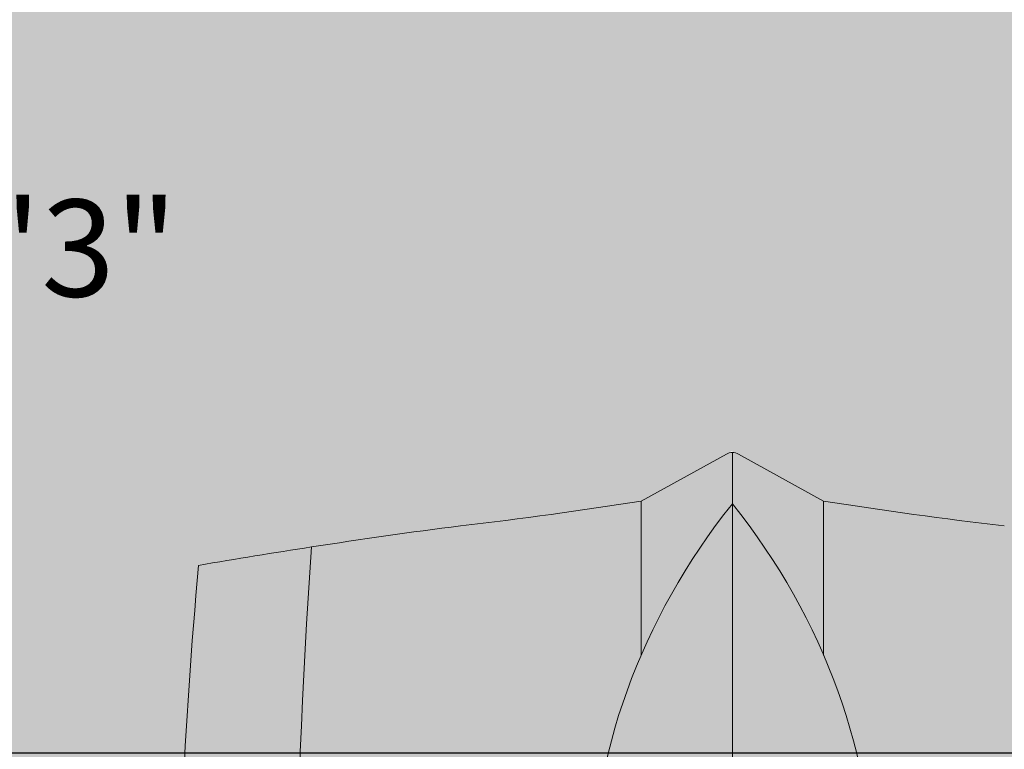
# Model space of a CAD drawing. Units: inches. Extents: x 389 to 971, y 148 to 870.
# Tile 2 of 14: x 477 to 529, y 389 to 428. Entities that reach past the tile are written whole.
import ezdxf

# ---------------------------------------------------------------- set-up
doc = ezdxf.new("R2010")
doc.units = ezdxf.units.IN
doc.header["$MEASUREMENT"] = 0
for name, color, linetype, lineweight in [('A-ANNO-DIMS', 2, 'Continuous', 18), ('A-AREA-IDEN', 7, 'Continuous', 18), ('C-VEHI', 8, 'Continuous', 13), ('L-GRND-BASE-PATT', 8, 'Continuous', 13)]:
    doc.layers.add(name, color=color, linetype=linetype, lineweight=lineweight)
doc.layers.add('C-VEHI-PATT', color=18, linetype='Continuous', lineweight=13, true_color=0x000000)
doc.layers.add('L-GRND-PATT', color=39, linetype='Continuous', lineweight=13, true_color=0x603913)
doc.styles.get("Standard").update_dxf_attribs({"font": 'arial.ttf'})
doc.dimstyles.get("Standard").update_dxf_attribs({"dimtxt": 8, "dimasz": 8, "dimexe": 0.18, "dimexo": 0.0625, "dimgap": 0.09, "dimtad": 0, "dimtih": 1, "dimtoh": 1, "dimdec": 0, "dimzin": 0, "dimdsep": 46, "dimlunit": 3, "dimtxsty": 'Standard', "dimcen": 0.09, "dimadec": 0, "dimazin": 0, "dimtfac": 1, "dimtdec": 0, "dimtofl": 0, "dimtmove": 0, "dimatfit": 3, "dimfxl": 1, "dimtolj": 1, "dimtzin": 0, "dimarcsym": 0})

# ---------------------------------------------------------------- blocks, each defined once
blk = doc.blocks.new('*U7')
for p, q in [((3.266462181856987, 6.128290093440767), (0.1022408397004821, 0.4060708604429806)), ((-4.43e-14, -2.558e-13), (51.68362801571248, -2.558e-13)), ((0.1022408397004821, -0.4060708604432933), (3.266462181856987, -6.128290093441194))]:
    blk.add_line(p, q)
for centre, major_axis, ratio, start_param, end_param in [((-204.4946649195746, 52.39684969293512), (4.12053e-11, -250.9602162198571), 0.8423038695441164, 1.385369446298923, 1.434372047871027), ((29.77279020470884, -46.66302566589627), (5.12e-14, 56.16885904951626), 0.842303869543976, 7e-16, 0.5903187773915901), ((0.6232400376122422, -1.421e-13), (1e-16, -0.7399230374541245), 0.842303869543842, 4.131459131953847, 5.293318828815531), ((29.77279020470884, 46.66302566589578), (4.004e-13, 56.16885904951626), 0.8423038695439734, 2.55127387619821, 3.141592653589801), ((-204.4946649195746, -52.39684969293552), (4.02945e-11, 250.9602162198562), 0.8423038695441192, -1.43437204787103, -1.385369446298926), ((259.1750197310694, 27.52442688365929), (1.08535e-11, 305.3028914629043), 0.8423038695439974, 1.721347632622872, 1.754579237318777), ((266.0300214172791, 27.52442688366566), (8.75241e-11, 313.3077612806533), 0.8423038695441819, 1.749832154434603, 1.774516663432659), ((37.47375371777847, 593.9621830607904), (1.1693e-12, -623.3282099673584), 0.8423038695439528, -0.0593185269054384, 0.0455465850287298), ((41.19115208863322, 490.8631038926152), (1.37757e-11, -528.2339998381949), 0.8423038695440652, -0.0755983031097181, -0.0028100083537155)]:
    blk.add_ellipse(centre, major_axis=major_axis, ratio=ratio, start_param=start_param, end_param=end_param)
blk = doc.blocks.new('*D53')
at = {"layer": 'A-ANNO-DIMS', "color": 0, "lineweight": -2, "transparency": 16777216}
for p, q in [((397.8910240000004, 396.9189020000002), (397.8910240000004, 404.9189020000001)), ((690.1535240000002, 388.9189020000003), (397.7110240000004, 388.9189020000002)), ((690.1535240000002, 376.9189020000001), (397.7110240000005, 376.9189020000001)), ((397.8910240000005, 368.9189020000001), (397.8910240000005, 360.918902))]:
    blk.add_line(p, q, dxfattribs=at)
at = {"layer": 'A-ANNO-DIMS', "color": 0, "transparency": 16777216}
for points in [[(396.5576906666671, 396.9189020000002), (399.2243573333337, 396.9189020000002), (397.8910240000004, 388.9189020000002)], [(396.5576906666671, 368.9189020000001), (399.2243573333338, 368.9189020000001), (397.8910240000005, 376.9189020000001)]]:
    blk.add_solid(points, dxfattribs=at)
at = {"layer": 'Defpoints', "color": 0, "transparency": 16777216}
for p in [(397.8910240000004, 388.9189020000002), (690.2160240000001, 388.9189020000003), (690.2160240000001, 376.9189020000001)]:
    blk.add_point(p, dxfattribs=at)
at = {"layer": 'A-ANNO-DIMS', "color": 0, "transparency": 16777216, "insert": (397.8910240000004, 382.9189019999999), "char_height": 8, "attachment_point": 5}
blk.add_mtext('\\A1;12', dxfattribs=at)

msp = doc.modelspace()

# ---------------------------------------------------------------- hatches: boundary and pattern name
at = {"layer": 'C-VEHI-PATT'}
h = msp.add_hatch(color=256, dxfattribs=at)
h.dxf.hatch_style = 1
edge = h.paths.add_edge_path()
edge.add_ellipse((550.9021553826709, 381.4331108862803), major_axis=(-43.99405423656321, 1.9369e-12), ratio=0.8423038695439613, start_angle=-29.43856959797762, end_angle=1.8189894035458565e-12, ccw=False)
edge.add_line((514.3535105156315, 402.059641051582), (514.3535105156315, 404.7525403567118))
edge.add_ellipse((514.3535105156316, 404.2643898676136), major_axis=(0.5795420236673633, 2e-16), ratio=0.8423038695437671, start_angle=90.00000000001334, end_angle=127.9331304598466)
edge.add_line((514.0354569934393, 404.6724605914631), (509.5535496243029, 402.1940957519602))
edge.add_ellipse((473.3138688667988, 564.9222417143382), major_axis=(196.5636751472093, 8.4793e-12), ratio=0.8423038695439335, start_angle=-80.7434339928015, end_angle=-77.44506735586577, ccw=False)
edge.add_ellipse((535.9119176052684, 201.7546502845751), major_axis=(239.1273775699096, 1.008988e-10), ratio=0.842303869543627, start_angle=100.2095389971183, end_angle=102.4446272934191)
edge.add_ellipse((979.5722266908713, 375.4013592680145), major_axis=(-488.2195497741742, 7.7268e-12), ratio=0.842303869543895, start_angle=-2.863714607837472, end_angle=2.198540565955285)
edge.add_ellipse((510.1338164488812, 299.4839331720496), major_axis=(70.3178640738586, 3.814e-12), ratio=0.8423038695439212, start_angle=94.08241069114638, end_angle=107.71995322274631, ccw=False)
edge.add_line((505.914122382133, 358.6062023341113), (522.79289864913, 358.606202334111))
edge.add_ellipse((518.5732045823792, 299.4839331720493), major_axis=(-70.31786407385354, 1.4408e-12), ratio=0.8423038695439844, start_angle=252.2800467772501, end_angle=265.91758930884987, ccw=False)
edge.add_ellipse((49.13479434038987, 375.4013592680261), major_axis=(-488.2195497741754, 2.5232e-12), ratio=0.8423038695439587, start_angle=177.8014594340444, end_angle=182.8637146078372)
edge.add_ellipse((492.795103425985, 201.7546502845724), major_axis=(239.12737756976, 4.82267e-11), ratio=0.8423038695441539, start_angle=77.5553727065425, end_angle=79.79046100284327)
edge.add_ellipse((555.3931521644682, 564.9222417143374), major_axis=(-196.5636751472384, 3.62381e-11), ratio=0.8423038695438114, start_angle=77.4450673558726, end_angle=80.74343399280832, ccw=False)
edge.add_line((519.1534714069603, 402.19409575196), (514.671564037824, 404.6724605914631))
edge.add_ellipse((514.3535105156316, 404.2643898676136), major_axis=(0.5795420236673633, 2e-16), ratio=0.8423038695437671, start_angle=52.06686954015338, end_angle=90.00000000001334)
edge.add_line((514.3535105156315, 404.7525403567118), (514.3535105156315, 402.0596410515821))
edge.add_ellipse((477.8048656485917, 381.4331108862812), major_axis=(-43.99405423656326, 6.67e-13), ratio=0.8423038695439753, start_angle=180.0000000000002, end_angle=209.4385695979796, ccw=False)
edge.add_line((521.7989198851549, 381.4331108862806), (521.7989198851549, 379.5923831537828))
edge.add_line((521.7989198851549, 379.5923831537828), (523.2258361412675, 379.5923831537828))
edge.add_ellipse((523.0896049791924, 379.1042326646847), major_axis=(0.5795420236669786, 3.601e-13), ratio=0.8423038695443263, start_angle=45.519789117397124, end_angle=89.99999999996442, ccw=False)
edge.add_line((523.4589887688404, 379.4803801228631), (527.8015488731598, 376.4548385069232))
edge.add_line((527.8015488731598, 376.4548385069232), (527.8015488731597, 364.8548231745798))
edge.add_ellipse((524.8002343791572, 364.9712406163019), major_axis=(0.279312372030448, 4.96584264291768), ratio=0.6038335755719146, start_angle=106.34259195429831, end_angle=270.9979857249735, ccw=False)
edge.add_line((521.7989198851548, 364.2715269884119), (521.7989198851549, 381.4331108862806))
edge.add_ellipse((477.8048656485917, 381.4331108862812), major_axis=(-43.99405423656326, 6.67e-13), ratio=0.8423038695439753, start_angle=180.0000000000001, end_angle=209.4385695979795)
edge.add_ellipse((550.9021553826709, 381.4331108862803), major_axis=(-43.99405423656321, 1.9369e-12), ratio=0.8423038695439613, start_angle=-29.43856959797755, end_angle=1.8539e-12)
edge.add_line((506.9081011461076, 381.43311088628), (506.9081011461074, 364.2715269884121))
edge.add_ellipse((503.9067866521049, 364.9712406163021), major_axis=(-0.2793123720310282, 4.965842642917721), ratio=0.6038335755718928, start_angle=89.00201427501901, end_angle=253.6574080456941, ccw=False)
edge.add_line((500.9054721581025, 364.8548231745812), (500.9054721581025, 376.4548385069235))
edge.add_line((500.9054721581025, 376.4548385069235), (505.3530060491612, 379.5535172937331))
edge.add_ellipse((505.61741605207, 379.1042326646849), major_axis=(-0.5795420236672051, 1.236e-13), ratio=0.842303869543997, start_angle=-89.99999999998778, end_angle=-45.51978911742469, ccw=False)
edge.add_line((505.61741605207, 379.5923831537831), (506.9081011461076, 379.5923831537831))
edge.add_line((506.9081011461076, 379.5923831537831), (506.9081011461076, 381.43311088628))
h = msp.add_hatch(color=256, dxfattribs=at)
h.dxf.hatch_style = 1
edge = h.paths.add_edge_path()
edge.add_ellipse((550.9021553826709, 381.4331108862803), major_axis=(-43.99405423656321, 1.9369e-12), ratio=0.8423038695439613, start_angle=-17.01851281727818, end_angle=1.8189894035458565e-12, ccw=False)
edge.add_line((509.5535496243029, 394.0892586662828), (509.5535496243029, 402.1940957519602))
edge.add_ellipse((473.3138688667988, 564.9222417143382), major_axis=(196.5636751472093, 8.4793e-12), ratio=0.8423038695439335, start_angle=-80.7434339928015, end_angle=-77.44506735586577, ccw=False)
edge.add_ellipse((535.9119176052684, 201.7546502845751), major_axis=(239.1273775699096, 1.008988e-10), ratio=0.842303869543627, start_angle=100.2095389971183, end_angle=102.4446272934191)
edge.add_ellipse((979.5722266908713, 375.4013592680145), major_axis=(-488.2195497741742, 7.7268e-12), ratio=0.842303869543895, start_angle=-2.863714607837472, end_angle=2.198540565955285)
edge.add_ellipse((510.1338164488812, 299.4839331720496), major_axis=(70.3178640738586, 3.814e-12), ratio=0.8423038695439212, start_angle=94.08241069114638, end_angle=107.71995322274631, ccw=False)
edge.add_line((505.914122382133, 358.6062023341113), (509.5535496243029, 358.6062023341112))
edge.add_line((509.5535496243029, 358.6062023341112), (509.5535496243029, 394.0892586662828))
edge.add_ellipse((550.9021553826709, 381.4331108862803), major_axis=(-43.99405423656321, 1.9369e-12), ratio=0.8423038695439613, start_angle=-17.01851281727824, end_angle=1.8539e-12)
edge.add_line((506.9081011461076, 381.43311088628), (506.9081011461074, 364.2715269884121))
edge.add_ellipse((503.9067866521049, 364.9712406163021), major_axis=(-0.2793123720310282, 4.965842642917721), ratio=0.6038335755718928, start_angle=89.00201427501901, end_angle=253.6574080456941, ccw=False)
edge.add_line((500.9054721581025, 364.8548231745812), (500.9054721581025, 376.4548385069235))
edge.add_line((500.9054721581025, 376.4548385069235), (505.3172273641584, 379.5285896248376))
edge.add_ellipse((505.61741605207, 379.1042326646849), major_axis=(-0.5795420236672051, 1.236e-13), ratio=0.842303869543997, start_angle=-89.99999999998778, end_angle=-45.51978911742469, ccw=False)
edge.add_line((505.61741605207, 379.5923831537831), (506.9081011461076, 379.5923831537831))
edge.add_line((506.9081011461076, 379.5923831537831), (506.9081011461076, 381.43311088628))
h = msp.add_hatch(color=256, dxfattribs=at)
h.dxf.hatch_style = 1
edge = h.paths.add_edge_path()
edge.add_ellipse((492.795103425985, 201.7546502845724), major_axis=(239.12737756976, 4.82267e-11), ratio=0.8423038695441539, start_angle=77.5553727065425, end_angle=79.79046100284327)
edge.add_ellipse((555.3931521644682, 564.9222417143374), major_axis=(-196.5636751472384, 3.62381e-11), ratio=0.8423038695438114, start_angle=77.4450673558726, end_angle=80.74343399280832, ccw=False)
edge.add_line((519.1534714069603, 402.19409575196), (519.1534714069603, 394.0892586662818))
edge.add_ellipse((477.8048656485917, 381.4331108862812), major_axis=(-43.99405423656326, 6.67e-13), ratio=0.8423038695439753, start_angle=180.0000000000002, end_angle=197.0185128172791, ccw=False)
edge.add_line((521.7989198851549, 381.4331108862806), (521.7989198851549, 379.5923831537828))
edge.add_line((521.7989198851549, 379.5923831537828), (523.1794038652976, 379.5923831537828))
edge.add_ellipse((523.0896049791924, 379.1042326646847), major_axis=(0.5795420236669786, 3.601e-13), ratio=0.8423038695443263, start_angle=45.519789117397124, end_angle=89.99999999996442, ccw=False)
edge.add_line((523.4589887688405, 379.480380122863), (527.8015488731598, 376.4548385069232))
edge.add_line((527.8015488731598, 376.4548385069232), (527.8015488731597, 364.8548231745798))
edge.add_ellipse((524.8002343791572, 364.9712406163019), major_axis=(0.279312372030448, 4.96584264291768), ratio=0.6038335755719146, start_angle=106.34259195429831, end_angle=270.9979857249735, ccw=False)
edge.add_line((521.7989198851548, 364.2715269884119), (521.7989198851549, 381.4331108862806))
edge.add_ellipse((477.8048656485917, 381.4331108862812), major_axis=(-43.99405423656326, 6.67e-13), ratio=0.8423038695439753, start_angle=180.0000000000001, end_angle=197.018512817279)
edge.add_line((519.1534714069603, 394.0892586662818), (519.1534714069603, 358.6062023341111))
edge.add_line((519.1534714069603, 358.6062023341111), (522.79289864913, 358.606202334111))
edge.add_ellipse((518.5732045823792, 299.4839331720493), major_axis=(-70.31786407385354, 1.4408e-12), ratio=0.8423038695439844, start_angle=252.2800467772501, end_angle=265.91758930884987, ccw=False)
edge.add_ellipse((49.13479434038987, 375.4013592680261), major_axis=(-488.2195497741754, 2.5232e-12), ratio=0.8423038695439587, start_angle=177.8014594340444, end_angle=182.8637146078372)
h = msp.add_hatch(color=256, dxfattribs=at)
h.dxf.hatch_style = 1
edge = h.paths.add_edge_path(flags=16)
edge.add_ellipse((3386.011413077446, 329.726312794031), major_axis=(-2896.629999631248, 1.069454e-10), ratio=0.8423038695494893, start_angle=-0.1208973690315247, end_angle=0.3640763488915013, ccw=False)
edge.add_line((489.3905023836935, 335.8383575186984), (486.2179253655185, 346.1978202249628))
edge.add_ellipse((8782.002602781096, 354.247254279773), major_axis=(-8295.790181758603, 9.87839e-10), ratio=0.8423038695486498, start_angle=0.0555943135052214, end_angle=0.3777641939157137)
edge.add_line((486.4665645878948, 299.5520931219791), (489.4638383140943, 311.3204429697198))
edge = h.paths.add_edge_path(flags=16)
edge.add_ellipse((512.1608573463288, 287.5825181681774), major_axis=(62.33048198263887, 2.0798e-12), ratio=0.8423038695439498, start_angle=94.8700695971331, end_angle=112.791914877584)
edge.add_line((491.3642517254777, 337.0752369161335), (489.6529508739416, 349.9015767089268))
edge.add_ellipse((510.1338164488795, 298.7862183048575), major_axis=(64.04807894948699, 3.9006e-12), ratio=0.8423038695439252, start_angle=94.27742096304979, end_angle=111.83495379670401, ccw=False)
edge.add_line((506.1068129054811, 352.6274231954524), (522.600208125781, 352.6274231954521))
edge.add_ellipse((518.5732045823798, 298.7862183048586), major_axis=(64.04807894948067, 3.24e-14), ratio=0.8423038695439885, start_angle=68.16504620328948, end_angle=85.72257903694378, ccw=False)
edge.add_line((539.05407015732, 349.9015767089259), (537.3427693057835, 337.0752369161327))
edge.add_ellipse((516.5461636849332, 287.5825181681899), major_axis=(62.33048198262021, 1.5954e-12), ratio=0.8423038695439995, start_angle=67.20808512240782, end_angle=85.12993040286212)
edge.add_line((521.0080028322477, 339.9490379899644), (507.6990181990146, 339.9490379899646))
edge = h.paths.add_edge_path(flags=16)
edge.add_ellipse((514.3535105156315, 391.3730654902235), major_axis=(-115.1512533244504, 1.8736e-12), ratio=0.8423038695439684, start_angle=76.4018653097696, end_angle=103.5981346902308)
edge.add_line((537.3427693057832, 296.3333211885938), (537.342769305783, 281.5897392316151))
edge.add_ellipse((514.3535105156313, 376.6294835332447), major_axis=(-115.1512533244486, 9.02e-13), ratio=0.8423038695439828, start_angle=76.40186530976922, end_angle=103.59813469023032, ccw=False)
edge.add_line((491.3642517254773, 281.5897392316156), (491.3642517254774, 296.3333211885945))
edge = h.paths.add_edge_path()
edge.add_ellipse((8782.002602781105, 354.2472542798386), major_axis=(-8296.949265805946, 5.39345e-11), ratio=0.8423038695428886, start_angle=0.3838667787920247, end_angle=0.5282714718170651)
edge.add_ellipse((8782.002602781105, 354.2472542798386), major_axis=(-8296.949265805946, 5.39345e-11), ratio=0.8423038695428886, start_angle=0.5282714718170651, end_angle=0.6465540970606384)
edge.add_ellipse((488.1158467995968, 260.6509346628684), major_axis=(2.318168094668909, 7.48e-14), ratio=0.8423038695439647, start_angle=180.6465540970884, end_angle=269.9999999999081)
edge.add_line((488.115846799593, 258.6983327064755), (491.3642517254771, 258.6983327064753))
edge.add_line((491.3642517254771, 258.6983327064753), (491.3642517254771, 274.201106836649))
edge.add_ellipse((493.6824198201462, 273.9438556676354), major_axis=(-2.318168094668919, 1.896e-13), ratio=0.8423038695439611, start_angle=-89.99999999999523, end_angle=4.718003765447065e-12, ccw=False)
edge.add_line((493.6824198201462, 275.8964576240284), (535.3300149439905, 275.8964576240277))
edge.add_ellipse((535.024601211114, 273.9438556676347), major_axis=(2.318168094668976, 2.946e-13), ratio=0.8423038695439647, start_angle=-7.275957614183426e-12, end_angle=89.99999999998943, ccw=False)
edge.add_line((537.342769305783, 273.9438556676347), (537.3427693057827, 258.698332706474))
edge.add_line((537.3427693057827, 258.698332706474), (540.591174231666, 258.6983327064739))
edge.add_ellipse((540.5911742316634, 260.6509346628669), major_axis=(-2.318168094668839, 2.143e-13), ratio=0.8423038695440144, start_angle=90.00000000008203, end_angle=179.3534459029346)
edge.add_ellipse((-7753.295581726658, 354.2472542799028), major_axis=(-8296.949265782761, 2.068448e-10), ratio=0.8423038695442414, start_angle=179.3534459029388, end_angle=179.3813568036815)
edge.add_ellipse((-7753.295581726658, 354.2472542799028), major_axis=(-8296.949265782761, 2.068448e-10), ratio=0.8423038695442414, start_angle=179.3813568036815, end_angle=179.4717285281828)
edge.add_ellipse((-7753.295581726658, 354.2472542799028), major_axis=(-8296.949265782761, 2.068448e-10), ratio=0.8423038695442414, start_angle=179.4717285281828, end_angle=179.6161332212082)
edge.add_ellipse((-7753.295581726658, 354.2472542799028), major_axis=(-8296.949265782761, 2.068448e-10), ratio=0.8423038695442414, start_angle=179.6161332212082, end_angle=180.090229088595)
edge.add_ellipse((-7753.295581726658, 354.2472542799028), major_axis=(-8296.949265782761, 2.068448e-10), ratio=0.8423038695442414, start_angle=180.090229088595, end_angle=180.134986576859)
edge.add_ellipse((129.8867725257751, 372.4897205359271), major_axis=(-413.7373561031673, 2.44623e-11), ratio=0.8423038695441432, start_angle=180.1806905311865, end_angle=182.1799503136479)
edge.add_ellipse((129.8867725257751, 372.4897205359271), major_axis=(-413.7373561031673, 2.44623e-11), ratio=0.8423038695441432, start_angle=182.1799503136479, end_angle=183.6504275857017)
edge.add_ellipse((492.7951034259847, 196.3854951855023), major_axis=(245.3971626940514, 1.422861e-10), ratio=0.8423038695444116, start_angle=76.21947101046817, end_angle=77.87403444768196)
edge.add_ellipse((49.13479434038987, 375.4013592680261), major_axis=(-488.2195497741754, 2.5232e-12), ratio=0.8423038695439587, start_angle=177.8014594340445, end_angle=182.8637146078372, ccw=False)
edge.add_ellipse((518.5732045823792, 299.4839331720493), major_axis=(-70.31786407385354, 1.4408e-12), ratio=0.8423038695439844, start_angle=252.2800467772501, end_angle=265.9175893088498)
edge.add_line((522.79289864913, 358.606202334111), (505.9141223821329, 358.6062023341113))
edge.add_ellipse((510.1338164488812, 299.4839331720496), major_axis=(70.3178640738586, 3.814e-12), ratio=0.8423038695439212, start_angle=94.08241069114636, end_angle=107.7199532227462)
edge.add_ellipse((979.5722266908713, 375.4013592680145), major_axis=(-488.2195497741742, 7.7268e-12), ratio=0.842303869543895, start_angle=-2.863714607837494, end_angle=2.198540565955284, ccw=False)
edge.add_ellipse((535.9119176052733, 196.3854951855018), major_axis=(-245.3971626940985, 1.013648e-10), ratio=0.8423038695442548, start_angle=-77.87403444769295, end_angle=-76.2194710104792)
edge.add_ellipse((898.8202485054873, 372.489720535918), major_axis=(413.7373561031672, 1.26113e-11), ratio=0.8423038695441164, start_angle=176.3495724142985, end_angle=177.8200496863523)
edge.add_ellipse((898.8202485054873, 372.489720535918), major_axis=(413.7373561031672, 1.26113e-11), ratio=0.8423038695441164, start_angle=177.8200496863523, end_angle=179.8643876095591)
edge.add_ellipse((8782.002602781105, 354.2472542798386), major_axis=(-8296.949265805946, 5.39345e-11), ratio=0.8423038695428886, start_angle=-0.1349865768573029, end_angle=-0.090229088593484)
edge.add_ellipse((8782.002602781105, 354.2472542798386), major_axis=(-8296.949265805946, 5.39345e-11), ratio=0.8423038695428886, start_angle=-0.090229088593484, end_angle=0.3838667787920247)
edge = h.paths.add_edge_path(flags=16)
edge.add_ellipse((-2357.304392046186, 329.7263127941099), major_axis=(2896.629999631251, 5.35614e-11), ratio=0.8423038695445265, start_angle=-0.3640763488920631, end_angle=0.1208973690309369)
edge.add_line((539.3165186475693, 335.8383575187012), (542.4890956657468, 346.1978202249727))
edge.add_ellipse((-7753.295581749842, 354.2472542800017), major_axis=(8295.790181758617, 3.2664368e-09), ratio=0.8423038695525207, start_angle=-0.37776419393310334, end_angle=-0.055594313522590255, ccw=False)
edge.add_line((542.240456443367, 299.5520931219743), (539.2431827171666, 311.3204429697195))
at = {"layer": 'L-GRND-BASE-PATT'}
h = msp.add_hatch(color=256, dxfattribs=at)
h.dxf.hatch_style = 1
edge = h.paths.add_edge_path(flags=16)
edge.add_ellipse((8782.002602781105, 354.2472542798386), major_axis=(-8296.949265805946, 5.39345e-11), ratio=0.8423038695428886, start_angle=-0.0902290885933894, end_angle=0.3838667787920258, ccw=False)
edge.add_ellipse((485.0533369751568, 368.2895347624687), major_axis=(-1.159084047334488, 1.838e-13), ratio=0.8423038695439892, start_angle=9.094947017729282e-12, end_angle=90.00000000000898, ccw=False)
edge.add_line((483.8942529278224, 368.2895347624687), (483.8942529278225, 387.6039063360424))
edge.add_ellipse((485.0533369751571, 387.2465553762829), major_axis=(1.159084047334488, 1.838e-13), ratio=0.8423038695439892, start_angle=89.99999999999102, end_angle=179.9999999999909, ccw=False)
edge.add_line((485.0533369751572, 388.2228563544795), (485.5047440247956, 388.2228563544795))
edge.add_ellipse((898.8202485054873, 372.489720535918), major_axis=(413.7373561031672, 1.26113e-11), ratio=0.8423038695441164, start_angle=176.3495724142986, end_angle=177.8200496863524, ccw=False)
edge.add_ellipse((535.9119176052733, 196.3854951855018), major_axis=(-245.3971626940985, 1.013648e-10), ratio=0.8423038695442548, start_angle=-77.87403444769302, end_angle=-76.2194710104792, ccw=False)
edge.add_ellipse((535.9119176052684, 201.7546502845751), major_axis=(239.1273775699096, 1.008988e-10), ratio=0.842303869543627, start_angle=100.20953899711827, end_angle=102.44462729341922, ccw=False)
edge.add_ellipse((473.3138688667988, 564.9222417143382), major_axis=(196.5636751472093, 8.4793e-12), ratio=0.8423038695439335, start_angle=-80.74343399280163, end_angle=-77.44506735586587)
edge.add_line((509.5535496243029, 402.1940957519602), (514.3535105156315, 404.8483349684994))
edge.add_line((514.3535105156315, 404.8483349684994), (514.3535105156315, 404.7971763262221))
edge.add_ellipse((514.3535105156316, 404.2643898676136), major_axis=(0.5795420236673633, 2e-16), ratio=0.8423038695437671, start_angle=52.06686954015339, end_angle=90.00000000001342, ccw=False)
edge.add_line((514.671564037824, 404.672460591463), (519.1534714069603, 402.19409575196))
edge.add_ellipse((555.3931521644682, 564.9222417143374), major_axis=(-196.5636751472384, 3.62381e-11), ratio=0.8423038695438114, start_angle=77.44506735587258, end_angle=80.74343399280833)
edge.add_ellipse((492.795103425985, 201.7546502845724), major_axis=(239.12737756976, 4.82267e-11), ratio=0.8423038695441539, start_angle=77.55537270654253, end_angle=79.7904610028433, ccw=False)
edge.add_ellipse((492.7951034259847, 196.3854951855023), major_axis=(245.3971626940514, 1.422861e-10), ratio=0.8423038695444116, start_angle=76.21947101046823, end_angle=77.87403444768199, ccw=False)
edge.add_ellipse((129.8867725257751, 372.4897205359271), major_axis=(-413.7373561031673, 2.44623e-11), ratio=0.8423038695441432, start_angle=182.179950313648, end_angle=183.6504275857018, ccw=False)
edge.add_line((543.2022770064673, 388.2228563544788), (544.0779382625514, 388.2228563544787))
edge.add_ellipse((543.6536840561057, 387.2465553762822), major_axis=(-1.159084047334545, 1.527e-13), ratio=0.8423038695438989, start_angle=180.0000000000075, end_angle=270.00000000000756, ccw=False)
edge.add_line((544.8127681034401, 387.2465553762826), (544.8127681034399, 367.9321838027083))
edge.add_ellipse((543.6536840561054, 368.2895347624679), major_axis=(1.159084047334544, 7.24e-14), ratio=0.8423038695439478, start_angle=269.9999999999964, end_angle=359.9999999999964, ccw=False)
edge.add_ellipse((-7753.295581726658, 354.2472542799028), major_axis=(-8296.949265782761, 2.068448e-10), ratio=0.8423038695442414, start_angle=179.6161332212083, end_angle=180.0902290885951, ccw=False)
edge.add_line((543.3912265319653, 298.6607849184036), (544.0779382625504, 298.6607849184036))
edge.add_ellipse((543.6536840561046, 297.6844839402071), major_axis=(1.159084047334431, 1.769e-13), ratio=0.8423038695439814, start_angle=-1.1482370609883219e-11, end_angle=89.99999999999119, ccw=False)
edge.add_line((544.8127681034391, 297.684483940207), (544.8127681034387, 278.3701123666333))
edge.add_ellipse((543.6536840561043, 278.727463326393), major_axis=(-1.159084047334431, 2.574e-13), ratio=0.8423038695440306, start_angle=90.00000000001268, end_angle=180.0000000000099, ccw=False)
edge.add_line((543.6536840561045, 277.7511623481965), (543.1566278692261, 277.7511623481965))
edge.add_ellipse((-7753.295581726658, 354.2472542799028), major_axis=(-8296.949265782761, 2.068448e-10), ratio=0.8423038695442414, start_angle=179.3813568036816, end_angle=179.4717285281829, ccw=False)
edge.add_ellipse((542.4236240941387, 263.2762864208561), major_axis=(-1.738626071001761, 2.132e-13), ratio=0.8423038695439151, start_angle=179.3717627838137, end_angle=248.464756601011, ccw=False)
edge.add_ellipse((-7753.875123750511, 354.2472542780016), major_axis=(-8298.740341433751, 2.4782644722e-06), ratio=0.8423038662721074, start_angle=179.3534459200609, end_angle=179.3717628008941, ccw=False)
edge.add_ellipse((540.0116322079951, 260.6509346628677), major_axis=(-4.109243751168186, 2.384e-13), ratio=0.842303869543976, start_angle=90.0000000000635, end_angle=179.3534459029233, ccw=False)
edge.add_line((540.0116322079991, 257.1897027503593), (488.6953888232593, 257.1897027503609))
edge.add_ellipse((488.6953888232669, 260.6509346628715), major_axis=(4.10924375117072, 1.262e-13), ratio=0.8423038695439824, start_angle=180.6465540970565, end_angle=269.9999999998589, ccw=False)
edge.add_ellipse((8782.582144816053, 354.2472542821698), major_axis=(-8298.740341477976, 1.8591886369e-06), ratio=0.8423038720186145, start_angle=0.6282372290784792, end_angle=0.6465541099116194, ccw=False)
edge.add_ellipse((486.2833969371199, 263.2762864208594), major_axis=(-1.738626071002378, 2.7e-13), ratio=0.8423038695439394, start_angle=-68.46475649596817, end_angle=0.6282372161796275, ccw=False)
edge.add_ellipse((8782.002602781105, 354.2472542798386), major_axis=(-8296.949265805946, 5.39345e-11), ratio=0.8423038695428886, start_angle=0.5282714718171064, end_angle=0.6465540970606867, ccw=False)
edge.add_line((485.5503931620382, 277.7511623481972), (484.6290827687102, 277.7511623481972))
edge.add_ellipse((485.0533369751559, 278.7274633263938), major_axis=(-1.159084047334545, 3.11e-13), ratio=0.8423038695439968, start_angle=1.5404566511278972e-11, end_angle=90.000000000012, ccw=False)
edge.add_line((483.8942529278214, 278.7274633263938), (483.8942529278216, 298.0418348999672))
edge.add_ellipse((485.053336975156, 297.6844839402078), major_axis=(1.159084047334488, 1.025e-13), ratio=0.8423038695440382, start_angle=89.99999999999488, end_angle=179.9999999999949, ccw=False)
edge = h.paths.add_edge_path(flags=0)
edge.add_ellipse((8782.002602781096, 354.247254279773), major_axis=(-8295.790181758603, 9.87839e-10), ratio=0.8423038695486498, start_angle=0.05559431350519617, end_angle=0.37776419391582294, ccw=False)
edge.add_line((486.2179253655185, 346.1978202249628), (489.3905023836935, 335.8383575186984))
edge.add_ellipse((3386.011413077446, 329.726312794031), major_axis=(-2896.629999631248, 1.069454e-10), ratio=0.8423038695494893, start_angle=-0.1208973690315206, end_angle=0.3640763488915184)
edge.add_line((489.4638383140943, 311.3204429697198), (486.4665645878948, 299.5520931219791))
edge = h.paths.add_edge_path(flags=0)
edge.add_ellipse((514.3535105156315, 391.3730654902235), major_axis=(-115.1512533244504, 1.8736e-12), ratio=0.8423038695439684, start_angle=76.4018653097696, end_angle=103.5981346902308)
edge.add_line((537.3427693057832, 296.3333211885938), (537.342769305783, 281.5897392316151))
edge.add_ellipse((514.3535105156313, 376.6294835332447), major_axis=(-115.1512533244486, 9.02e-13), ratio=0.8423038695439828, start_angle=76.40186530976922, end_angle=103.59813469023032, ccw=False)
edge.add_line((491.3642517254773, 281.5897392316156), (491.3642517254774, 296.3333211885945))
edge = h.paths.add_edge_path(flags=0)
edge.add_line((491.3642517254777, 337.0752369161334), (489.6529508739416, 349.9015767089268))
edge.add_ellipse((510.1338164488795, 298.7862183048575), major_axis=(64.04807894948699, 3.9006e-12), ratio=0.8423038695439252, start_angle=94.27742096304979, end_angle=111.83495379670401, ccw=False)
edge.add_line((506.106812905481, 352.6274231954524), (522.600208125781, 352.6274231954521))
edge.add_ellipse((518.5732045823798, 298.7862183048586), major_axis=(64.04807894948067, 3.24e-14), ratio=0.8423038695439885, start_angle=68.16504620328948, end_angle=85.72257903694378, ccw=False)
edge.add_line((539.05407015732, 349.9015767089259), (537.3427693057835, 337.0752369161327))
edge.add_ellipse((516.5461636849332, 287.5825181681899), major_axis=(62.33048198262021, 1.5954e-12), ratio=0.8423038695439995, start_angle=67.20808512240782, end_angle=85.12993040286212)
edge.add_line((521.0080028322477, 339.9490379899644), (507.6990181990146, 339.9490379899646))
edge.add_ellipse((512.1608573463288, 287.5825181681774), major_axis=(62.33048198263887, 2.0798e-12), ratio=0.8423038695439498, start_angle=94.8700695971331, end_angle=112.791914877584)
edge = h.paths.add_edge_path(flags=0)
edge.add_ellipse((493.6824198201462, 273.9438556676354), major_axis=(-2.318168094668919, 1.896e-13), ratio=0.8423038695439611, start_angle=-89.99999999999523, end_angle=4.718003765447065e-12, ccw=False)
edge.add_line((493.6824198201462, 275.8964576240284), (535.3743409680425, 275.8964576240277))
edge.add_ellipse((535.024601211114, 273.9438556676347), major_axis=(2.318168094668976, 2.946e-13), ratio=0.8423038695439647, start_angle=-7.275957614183426e-12, end_angle=89.99999999998943, ccw=False)
edge.add_line((537.342769305783, 273.9438556676347), (537.3427693057827, 258.698332706474))
edge.add_line((537.3427693057827, 258.698332706474), (540.5911742316662, 258.6983327064739))
edge.add_ellipse((540.5911742316634, 260.6509346628669), major_axis=(-2.318168094668839, 2.143e-13), ratio=0.8423038695440144, start_angle=90.00000000008203, end_angle=179.3534459029346)
edge.add_line((540.5911742316662, 258.6983327064739), (487.7691399811528, 258.6983327064755))
edge.add_ellipse((488.1158467995968, 260.6509346628684), major_axis=(2.318168094668909, 7.48e-14), ratio=0.8423038695439647, start_angle=180.6465540970884, end_angle=269.9999999999081)
edge.add_line((488.1158467995931, 258.6983327064755), (491.3642517254771, 258.6983327064754))
edge.add_line((491.3642517254771, 258.6983327064754), (491.3642517254771, 274.2384428182294))
h.paths.add_polyline_path([(746.1375687288224, 327.3223047166553), (750.1400147212453, 327.3223047166553), (750.1400147212453, 326.2830696147227), (798.1693712998389, 326.2830696147227), (798.1693712998389, 327.3223047166553), (802.1718172922616, 327.3223047166553), (802.1718172922616, 309.9783792024682, -0.1904762075443491), (746.1375687288224, 309.9783668090107)], flags=16)
h.paths.add_polyline_path([(782.1595875801748, 313.5684994305933), (782.1595893317732, 309.0414930416419, -0.0496282101666581), (766.1497986905329, 309.0414910503953), (766.1498004421323, 313.5684994305933)], flags=0)
h.paths.add_polyline_path([(755.1858908233534, 344.9352232902417), (755.1858908233534, 373.916311072083), (788.1243995226009, 373.916311072083), (788.1243995226009, 344.9352232902417)], flags=16)
h.paths.add_polyline_path([(757.1858908233535, 346.9352232902417), (757.1858908233535, 371.916311072083), (786.1243995226009, 371.916311072083), (786.1243995226009, 346.9352232902417)], flags=0)
h.paths.add_polyline_path([(803.6445810111745, 338.4878931208803), (803.6445810111745, 342.4903391133031), (804.6838161131072, 342.4903391133031), (804.6838161131072, 390.5196956918968), (803.6445810111748, 390.5196956918968), (803.6445810111748, 394.5221416843196), (820.9885065253617, 394.5221416843196, -0.1904762075443491), (820.9885189188192, 338.4878931208803)], flags=16)
h.paths.add_polyline_path([(806.8706930931005, 326.6963103558256), (806.4254411777042, 327.1415622712219), (806.4723791864895, 326.6297175483474)], flags=16)
h.paths.add_polyline_path([(822.0328146004263, 317.4007976138144), (822.1941503181826, 317.8932883068639), (821.562628166435, 317.9885306563034)], flags=16)
h.paths.add_polyline_path([(817.3983862972365, 358.5001248341902), (817.3983862972365, 374.5099119722327), (821.9253926861879, 374.5099137238312, -0.049628210166658), (821.9253946774346, 358.5001230825909)], flags=0)
h.paths.add_polyline_path([(808.1446344648577, 418.9736619306146), (808.2246858861593, 418.5632188717996), (808.5395491501399, 418.5787472453325)], flags=16)
h.paths.add_polyline_path([(820.3158762739024, 412.6690288868844), (820.4772119916585, 413.161519579934), (819.8456898399113, 413.2567619293735)], flags=16)
h.paths.add_polyline_path([(466.3155093563569, 235.5246322146605), (517.3806533266912, 235.5246322146605), (517.3806533266912, 244.4269231682286), (466.3155093563569, 244.4269231682286)], flags=24)
h.paths.add_polyline_path([(739.8737195480014, 256.2000079819968), (815.4040239338423, 256.2000079819968), (815.4040239338423, 265.3453807094367), (739.8737195480014, 265.3453807094367)], flags=24)
h.paths.add_polyline_path([(750.6081538187397, 393.6666679930368), (791.5680640722773, 393.6666679930368), (791.5680640722773, 412.3933175868746), (750.6081538187397, 412.3933175868746)], flags=24)
h.paths.add_polyline_path([(438.9630812812552, 410.0618566955462), (484.6203810968238, 410.0618566955462), (484.6203810968238, 429.1217352891893), (438.9630812812552, 429.1217352891893)], flags=24)
edge = h.paths.add_edge_path()
edge.add_line((839.2160244416713, 285.6445131961097), (611.8786784019748, 285.6445131961099))
edge.add_line((611.8786784019748, 285.6445131961099), (604.3870116090119, 285.6445131961097))
edge.add_line((604.3870116090119, 285.6445131961097), (595.3870116090119, 285.6445131961097))
edge.add_line((595.3870116090119, 285.6445131961097), (595.3870116090118, 370.1553848722774))
edge.add_line((595.3870116090118, 370.1553848722774), (604.0816928471932, 370.1553848722774))
edge.add_line((604.0816928471932, 370.1553848722774), (604.0816928471932, 371.3788335667469))
edge.add_line((604.0816928471932, 371.3788335667469), (632.0194586761203, 371.3788335667469))
edge.add_arc((604.0816928471932, 370.1553848722773), 27.96454158787471, 2.507490703587644, 90.00000000000003)
edge.add_line((604.0816928471932, 398.1199264601519), (599.8870116090108, 398.1652144688576))
edge.add_line((599.8870116090108, 398.1652144688576), (604.4225424425357, 398.1652144688576))
edge.add_arc((604.4225424425357, 428.4020866923496), 30.23687222349201, 270.0000000000002, 357.492509296413)
edge.add_line((634.6304631740308, 427.0792235325719), (604.4225424425357, 427.0792235325719))
edge.add_line((604.4225424425357, 427.0792235325719), (604.4225424425357, 428.4020866923497))
edge.add_line((604.4225424425357, 428.4020866923497), (599.8870116090119, 428.4020866923497))
edge.add_line((599.8870116090119, 428.4020866923497), (595.3870116090116, 428.4020866923497))
edge.add_line((595.3870116090116, 428.4020866923497), (595.3870116090118, 434.6445131961097))
edge.add_line((595.3870116090118, 434.6445131961097), (585.0790669792458, 434.6445131961097))
edge.add_line((585.0790669792458, 434.6445131961097), (540.3921730610418, 434.6445131961097))
edge.add_line((540.3921730610418, 434.6445131961097), (526.712508448134, 434.6445131961097))
edge.add_line((526.712508448134, 434.6445131961097), (488.4094553949635, 434.6445131961097))
edge.add_line((488.4094553949635, 434.6445131961097), (432.2160244416713, 434.6445131961097))
edge.add_line((432.2160244416713, 434.6445131961097), (432.2160244416713, 243.6445131961098))
edge.add_line((432.2160244416713, 243.6445131961098), (437.2160244416714, 243.6445131961098))
edge.add_line((437.2160244416714, 243.6445131961098), (437.2160244416714, 234.6445131961098))
edge.add_line((437.2160244416714, 234.6445131961098), (581.2160244416713, 234.6445131961098))
edge.add_line((581.2160244416713, 234.6445131961098), (581.2160244416713, 238.6445131961097))
edge.add_line((581.2160244416713, 238.6445131961097), (581.2160244416713, 243.6445131961098))
edge.add_line((581.2160244416713, 243.6445131961098), (590.2160244416713, 243.6445131961098))
edge.add_line((590.2160244416713, 243.6445131961098), (590.2160244416713, 238.6445131961097))
edge.add_line((590.2160244416713, 238.6445131961097), (839.2160244416713, 238.6445131961098))
edge.add_line((839.2160244416713, 238.6445131961098), (839.2160244416713, 285.6445131961097))
at = {"layer": 'L-GRND-PATT'}
h = msp.add_hatch(dxfattribs=at)
h.set_pattern_fill('EARTH', color=256, angle=45)
h.set_pattern_definition([(45, (0, 0), (0, 8.980256121069154), [6.349999999999999, -6.349999999999999]), (45, (-1.683798022700466, 1.683798022700466), (0, 8.980256121069154), [6.349999999999999, -6.349999999999999]), (45, (-3.367596045400933, 3.367596045400933), (0, 8.980256121069154), [6.349999999999999, -6.349999999999999]), (135, (-3.367596045400933, 4.490128060534576), (-8.980256121069154, 0), [6.349999999999999, -6.349999999999999]), (135, (-1.683798022700466, 6.173926083235043), (-8.980256121069154, 0), [6.349999999999999, -6.349999999999999]), (135, (0, 7.85772410593551), (-8.980256121069154, 0), [6.349999999999999, -6.349999999999999])])
h.paths.add_polyline_path([(432.2160244416713, 243.6445131961098), (437.2160244416714, 243.6445131961098), (437.2160244416714, 234.6445131961098), (581.2160244416713, 234.6445131961098), (581.2160244416713, 238.6445131961097), (581.2160244416713, 243.6445131961098), (590.2160244416713, 243.6445131961098), (590.2160244416713, 238.6445131961097), (839.2160244416713, 238.6445131961098), (839.2160244416712, 285.6445131961097), (810.0513609197296, 285.6445131961097), (733.8056934525983, 285.6445131961099), (684.2433676403508, 285.6445131961098), (611.8786784019748, 285.6445131961099), (604.3870116090119, 285.6445131961097), (595.3870116090119, 285.6445131961097), (595.3870116090118, 370.1553848722774), (604.0816928471932, 370.1553848722774), (604.0816928471932, 371.3788335667469), (632.0194586761203, 371.3788335667469, 0.4014527144963568), (604.0816928471932, 398.119926460152), (599.8870116090127, 398.1652144688576), (604.4225424425357, 398.1652144688576, 0.4014527144963579), (634.6304631740308, 427.0792235325719), (604.4225424425357, 427.0792235325719), (604.4225424425357, 428.4020866923497), (599.8870116090119, 428.4020866923497), (595.3870116090116, 428.4020866923497), (595.3870116090118, 434.6445131961097), (585.0790669792458, 434.6445131961097), (540.3921730610418, 434.6445131961097), (526.712508448134, 434.6445131961097), (488.4094553949635, 434.6445131961097), (432.2160244416713, 434.6445131961097)])
edge = h.paths.add_edge_path(flags=16)
edge.add_line((483.8942529278214, 278.7274633263938), (483.8942529278216, 298.2563878122772))
edge.add_ellipse((485.053336975156, 297.6844839402078), major_axis=(1.159084047334488, 1.025e-13), ratio=0.8423038695440382, start_angle=89.99999999999488, end_angle=179.9999999999949, ccw=False)
edge.add_ellipse((8782.002602781105, 354.2472542798386), major_axis=(-8296.949265805946, 5.39345e-11), ratio=0.8423038695428886, start_angle=-0.0902290885933894, end_angle=0.3838667787920258, ccw=False)
edge.add_ellipse((485.0533369751568, 368.2895347624687), major_axis=(-1.159084047334488, 1.838e-13), ratio=0.8423038695439892, start_angle=9.094947017729282e-12, end_angle=90.00000000000898, ccw=False)
edge.add_line((483.8942529278224, 368.2895347624687), (483.8942529278225, 387.8184592483523))
edge.add_ellipse((485.0533369751571, 387.2465553762829), major_axis=(1.159084047334488, 1.838e-13), ratio=0.8423038695439892, start_angle=89.99999999999102, end_angle=179.9999999999909, ccw=False)
edge.add_ellipse((898.8202485054873, 372.489720535918), major_axis=(413.7373561031672, 1.26113e-11), ratio=0.8423038695441164, start_angle=176.3495724142986, end_angle=177.8200496863524, ccw=False)
edge.add_ellipse((535.9119176052733, 196.3854951855018), major_axis=(-245.3971626940985, 1.013648e-10), ratio=0.8423038695442548, start_angle=-77.87403444769302, end_angle=-76.2194710104792, ccw=False)
edge.add_ellipse((535.9119176052684, 201.7546502845751), major_axis=(239.1273775699096, 1.008988e-10), ratio=0.842303869543627, start_angle=100.20953899711827, end_angle=102.44462729341922, ccw=False)
edge.add_ellipse((473.3138688667988, 564.9222417143382), major_axis=(196.5636751472093, 8.4793e-12), ratio=0.8423038695439335, start_angle=-80.74343399280163, end_angle=-77.44506735586587)
edge.add_line((509.5535496243029, 402.1940957519602), (514.3535105156316, 404.8483349684994))
edge.add_line((514.3535105156316, 404.8483349684994), (519.1534714069603, 402.19409575196))
edge.add_ellipse((555.3931521644682, 564.9222417143374), major_axis=(-196.5636751472384, 3.62381e-11), ratio=0.8423038695438114, start_angle=77.44506735587258, end_angle=80.74343399280833)
edge.add_ellipse((492.795103425985, 201.7546502845724), major_axis=(239.12737756976, 4.82267e-11), ratio=0.8423038695441539, start_angle=77.55537270654253, end_angle=79.7904610028433, ccw=False)
edge.add_ellipse((492.7951034259847, 196.3854951855023), major_axis=(245.3971626940514, 1.422861e-10), ratio=0.8423038695444116, start_angle=76.21947101046823, end_angle=77.87403444768199, ccw=False)
edge.add_ellipse((129.8867725257751, 372.4897205359271), major_axis=(-413.7373561031673, 2.44623e-11), ratio=0.8423038695441432, start_angle=182.179950313648, end_angle=183.6504275857018, ccw=False)
edge.add_line((543.2022770064673, 388.2228563544789), (544.3326597711041, 388.2228563544786))
edge.add_ellipse((543.6536840561057, 387.2465553762822), major_axis=(-1.159084047334545, 1.527e-13), ratio=0.8423038695438989, start_angle=180.0000000000075, end_angle=270.00000000000756, ccw=False)
edge.add_line((544.8127681034401, 387.2465553762825), (544.8127681034399, 367.7176308903986))
edge.add_ellipse((543.6536840561054, 368.2895347624679), major_axis=(1.159084047334544, 7.24e-14), ratio=0.8423038695439478, start_angle=269.9999999999964, end_angle=359.9999999999964, ccw=False)
edge.add_ellipse((-7753.295581726658, 354.2472542799028), major_axis=(-8296.949265782761, 2.068448e-10), ratio=0.8423038695442414, start_angle=179.6161332212083, end_angle=180.0902290885951, ccw=False)
edge.add_ellipse((543.6536840561046, 297.6844839402071), major_axis=(1.159084047334431, 1.769e-13), ratio=0.8423038695439814, start_angle=-1.1482370609883219e-11, end_angle=89.99999999999119, ccw=False)
edge.add_line((544.8127681034391, 297.6844839402071), (544.8127681034387, 278.1555594543235))
edge.add_ellipse((543.6536840561043, 278.727463326393), major_axis=(-1.159084047334431, 2.574e-13), ratio=0.8423038695440306, start_angle=90.00000000001268, end_angle=180.0000000000099, ccw=False)
edge.add_ellipse((-7753.295581726658, 354.2472542799028), major_axis=(-8296.949265782761, 2.068448e-10), ratio=0.8423038695442414, start_angle=179.3813568036816, end_angle=179.4717285281829, ccw=False)
edge.add_ellipse((542.4236240941387, 263.2762864208561), major_axis=(-1.738626071001761, 2.132e-13), ratio=0.8423038695439151, start_angle=179.3717627838137, end_angle=248.464756601011, ccw=False)
edge.add_ellipse((-7753.875123750511, 354.2472542780016), major_axis=(-8298.740341433751, 2.4782644722e-06), ratio=0.8423038662721074, start_angle=179.3534459200609, end_angle=179.3717628008941, ccw=False)
edge.add_ellipse((540.0116322079951, 260.6509346628677), major_axis=(-4.109243751168186, 2.384e-13), ratio=0.842303869543976, start_angle=90.0000000000635, end_angle=179.3534459029233, ccw=False)
edge.add_line((540.0116322079989, 257.1897027503593), (488.0808074948215, 257.1897027503609))
edge.add_ellipse((488.6953888232669, 260.6509346628715), major_axis=(4.10924375117072, 1.262e-13), ratio=0.8423038695439824, start_angle=180.6465540970565, end_angle=269.9999999998589, ccw=False)
edge.add_ellipse((8782.582144816053, 354.2472542821698), major_axis=(-8298.740341477976, 1.8591886369e-06), ratio=0.8423038720186145, start_angle=0.6282372290784792, end_angle=0.6465541099116194, ccw=False)
edge.add_ellipse((486.2833969371199, 263.2762864208594), major_axis=(-1.738626071002378, 2.7e-13), ratio=0.8423038695439394, start_angle=-68.46475649596817, end_angle=0.6282372161796275, ccw=False)
edge.add_ellipse((8782.002602781105, 354.2472542798386), major_axis=(-8296.949265805946, 5.39345e-11), ratio=0.8423038695428886, start_angle=0.5282714718171064, end_angle=0.6465540970606867, ccw=False)
edge.add_line((485.5503931620382, 277.7511623481972), (484.3743612601578, 277.7511623481972))
edge.add_ellipse((485.0533369751559, 278.7274633263938), major_axis=(-1.159084047334545, 3.11e-13), ratio=0.8423038695439968, start_angle=1.5404566511278972e-11, end_angle=90.000000000012, ccw=False)
edge = h.paths.add_edge_path(flags=0)
edge.add_ellipse((488.1158467995968, 260.6509346628684), major_axis=(2.318168094668909, 7.48e-14), ratio=0.8423038695439647, start_angle=180.6465540970884, end_angle=269.9999999999081)
edge.add_line((488.1158467995933, 258.6983327064755), (491.3642517254771, 258.6983327064753))
edge.add_line((491.3642517254771, 258.6983327064753), (491.3642517254771, 274.4686391213292))
edge.add_ellipse((493.6824198201462, 273.9438556676354), major_axis=(-2.318168094668919, 1.896e-13), ratio=0.8423038695439611, start_angle=-89.99999999999523, end_angle=4.718003765447065e-12, ccw=False)
edge.add_line((493.6824198201462, 275.8964576240284), (535.6476346230087, 275.8964576240277))
edge.add_ellipse((535.024601211114, 273.9438556676347), major_axis=(2.318168094668976, 2.946e-13), ratio=0.8423038695439647, start_angle=-7.275957614183426e-12, end_angle=89.99999999998943, ccw=False)
edge.add_line((537.342769305783, 273.9438556676347), (537.3427693057827, 258.698332706474))
edge.add_line((537.3427693057827, 258.698332706474), (541.2086129152347, 258.6983327064739))
edge.add_ellipse((540.5911742316634, 260.6509346628669), major_axis=(-2.318168094668839, 2.143e-13), ratio=0.8423038695440144, start_angle=90.00000000008203, end_angle=179.3534459029347, ccw=False)
edge.add_line((540.5911742316662, 258.6983327064739), (487.4984081160257, 258.6983327064755))
edge = h.paths.add_edge_path(flags=0)
edge.add_line((491.3642517254773, 281.5897392316156), (491.3642517254774, 296.3333211885945))
edge.add_ellipse((514.3535105156315, 391.3730654902235), major_axis=(-115.1512533244504, 1.8736e-12), ratio=0.8423038695439684, start_angle=76.4018653097696, end_angle=103.5981346902308)
edge.add_line((537.3427693057832, 296.3333211885938), (537.342769305783, 281.5897392316151))
edge.add_ellipse((514.3535105156313, 376.6294835332447), major_axis=(-115.1512533244486, 9.02e-13), ratio=0.8423038695439828, start_angle=76.40186530976922, end_angle=103.59813469023032, ccw=False)
edge = h.paths.add_edge_path(flags=0)
edge.add_ellipse((8782.002602781096, 354.247254279773), major_axis=(-8295.790181758603, 9.87839e-10), ratio=0.8423038695486498, start_angle=0.05559431350519617, end_angle=0.37776419391582294, ccw=False)
edge.add_line((486.2179253655185, 346.1978202249628), (489.3905023836935, 335.8383575186985))
edge.add_ellipse((3386.011413077446, 329.726312794031), major_axis=(-2896.629999631248, 1.069454e-10), ratio=0.8423038695494893, start_angle=-0.1208973690315206, end_angle=0.3640763488915184)
edge.add_line((489.4638383140943, 311.3204429697198), (486.4665645878948, 299.5520931219782))
edge = h.paths.add_edge_path(flags=0)
edge.add_line((491.3642517254777, 337.0752369161334), (489.6529508739416, 349.9015767089268))
edge.add_ellipse((510.1338164488795, 298.7862183048575), major_axis=(64.04807894948699, 3.9006e-12), ratio=0.8423038695439252, start_angle=94.27742096304979, end_angle=111.83495379670401, ccw=False)
edge.add_line((506.106812905481, 352.6274231954524), (522.600208125781, 352.6274231954521))
edge.add_ellipse((518.5732045823798, 298.7862183048586), major_axis=(64.04807894948067, 3.24e-14), ratio=0.8423038695439885, start_angle=68.16504620328948, end_angle=85.72257903694378, ccw=False)
edge.add_line((539.05407015732, 349.9015767089259), (537.3427693057835, 337.0752369161327))
edge.add_ellipse((516.5461636849332, 287.5825181681899), major_axis=(62.33048198262021, 1.5954e-12), ratio=0.8423038695439995, start_angle=67.20808512240782, end_angle=85.12993040286212)
edge.add_line((521.0080028322477, 339.9490379899644), (507.6990181990145, 339.9490379899646))
edge.add_ellipse((512.1608573463288, 287.5825181681774), major_axis=(62.33048198263887, 2.0798e-12), ratio=0.8423038695439498, start_angle=94.8700695971331, end_angle=112.791914877584)
h.paths.add_polyline_path([(466.3155093563569, 235.5246322146605), (517.3806533266912, 235.5246322146605), (517.3806533266912, 244.4269231682286), (466.3155093563569, 244.4269231682286)], flags=24)
h.paths.add_polyline_path([(739.8737195480014, 256.2000079819968), (815.4040239338423, 256.2000079819968), (815.4040239338423, 265.3453807094367), (739.8737195480014, 265.3453807094367)], flags=24)
h.paths.add_polyline_path([(438.9630812812552, 410.0618566955462), (484.6203810968238, 410.0618566955462), (484.6203810968238, 429.1217352891893), (438.9630812812552, 429.1217352891893)], flags=24)

# ---------------------------------------------------------------- linework, layer by layer
at = {"layer": 'C-VEHI'}
for p, q in [((509.5535496243029, 402.1940957519602), (509.5535496243029, 394.0892586662828)), ((519.1534714069603, 402.19409575196), (519.1534714069603, 394.0892586662819))]:
    msp.add_line(p, q, dxfattribs=at)

# ---------------------------------------------------------------- block references
at = {"layer": 'C-VEHI', "xscale": 0.7832463571634928, "yscale": 0.7832463571634928, "zscale": 0.7832463571634928, "rotation": 269.9999999999993}
msp.add_blockref('*U7', (514.3535105156318, 404.7525403567118), dxfattribs=at)

# ---------------------------------------------------------------- texts
at = {"layer": 'A-AREA-IDEN', "insert": (441.017032612244, 426.5799922935042), "char_height": 5.107875574604968, "attachment_point": 1}
msp.add_mtext_dynamic_manual_height_columns('  PARKING\\P13\'10" x 15\'3"', width=115.9269957180866, gutter_width=25.53937787302484, heights=[0], dxfattribs=at)

# ---------------------------------------------------------------- dimensions: what is measured, and where the dimension line sits
at = {"layer": 'A-ANNO-DIMS'}
dim = msp.add_linear_dim(base=(397.8910240000004, 388.9189020000002), p1=(690.216024, 376.918902), p2=(690.216024, 388.918902), angle=90, dimstyle='Standard', override={"dimdec": 0, "dimlfac": 1, "dimrnd": 0, "dimzin": 0, "dimdsep": 46, "dimlunit": 2}, dxfattribs=at)
dim.commit()
dim.dimension.update_dxf_attribs({"geometry": '*D53', "text_midpoint": (397.8910240000004, 382.9189019999999)})

doc.saveas('drawing.dxf')
